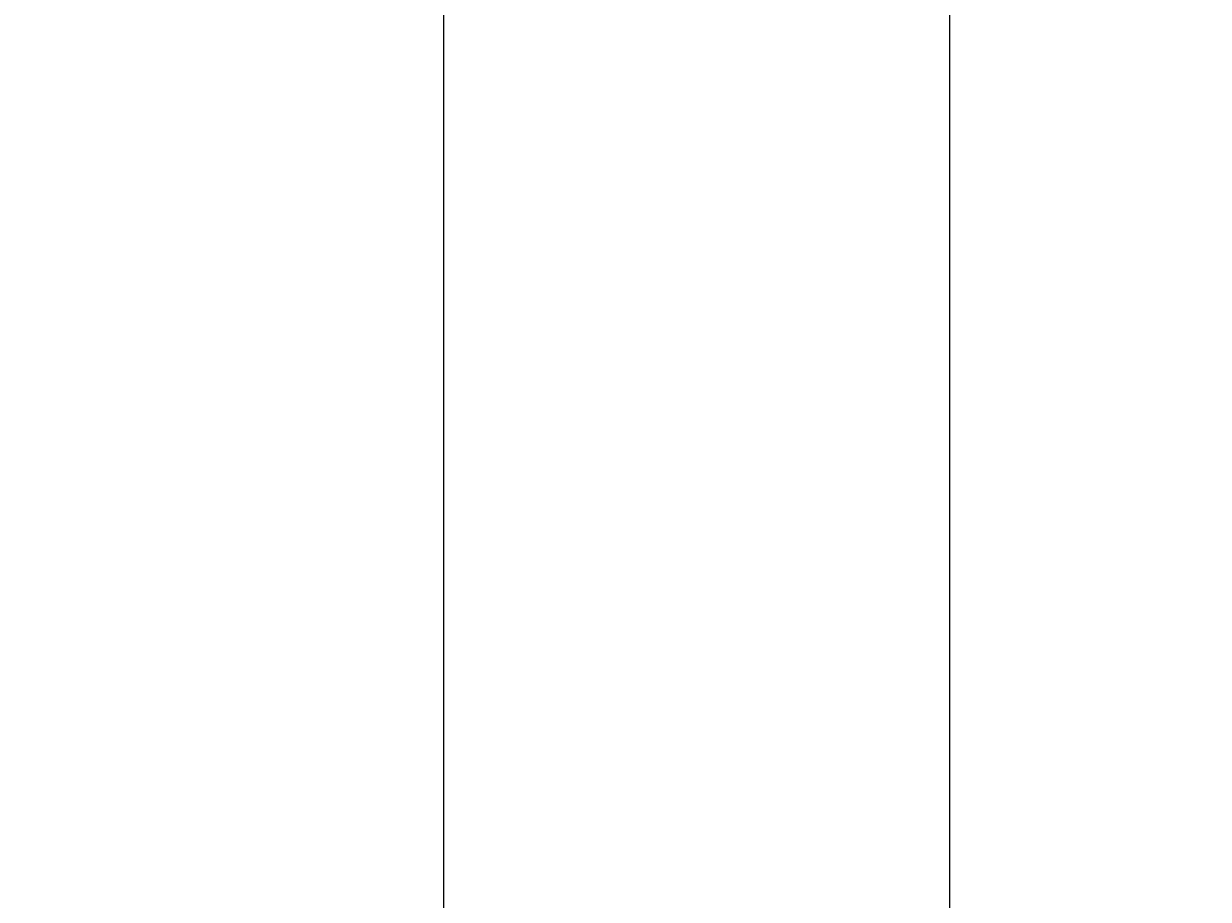
# Model space of a CAD drawing. Units: millimetres. Extents: x 19292 to 100733, y 12374 to 26974.
# Tile 6 of 24: x 29402 to 29589, y 15391 to 15530. Entities that reach past the tile are written whole.
import ezdxf

# ---------------------------------------------------------------- set-up
doc = ezdxf.new("R2010")
doc.units = ezdxf.units.MM
doc.layers.add('A-ANNO-DIMS', color=2, linetype='Continuous', lineweight=18)
doc.layers.add('A-DOOR', color=4, linetype='Continuous', lineweight=25)
doc.styles.get("Standard").update_dxf_attribs({"font": 'arial.ttf'})
doc.dimstyles.get("Standard").update_dxf_attribs({"dimtxt": 0.18, "dimasz": 0.18, "dimexe": 0.18, "dimexo": 0.0625, "dimgap": 0.09, "dimtad": 0, "dimtih": 1, "dimtoh": 1, "dimdec": 4, "dimzin": 0, "dimdsep": 46, "dimtxsty": 'Standard', "dimcen": 0.09, "dimadec": 0, "dimazin": 0, "dimtfac": 1, "dimtdec": 4, "dimtofl": 0, "dimtmove": 0, "dimatfit": 3, "dimfxl": 1, "dimtolj": 1, "dimtzin": 0, "dimarcsym": 0})

# ---------------------------------------------------------------- blocks, each defined once
blk = doc.blocks.new('*D79')
at = {"layer": 'A-ANNO-DIMS', "color": 0, "lineweight": -2, "transparency": 16777216}
for p, q in [((22694.13, 22860.66), (22694.13, 12808.81)), ((36144.17, 15985.66), (36144.17, 12808.81)), ((22694.31, 12808.99), (29418.73, 12808.99)), ((36143.99, 12808.99), (29419.57, 12808.99))]:
    blk.add_line(p, q, dxfattribs=at)
at = {"layer": 'A-ANNO-DIMS', "color": 0, "transparency": 16777216}
for points in [[(22694.31, 12809.02), (22694.31, 12808.96), (22694.13, 12808.99)], [(36143.99, 12809.02), (36143.99, 12808.96), (36144.17, 12808.99)]]:
    blk.add_solid(points, dxfattribs=at)
at = {"layer": 'Defpoints', "color": 0, "transparency": 16777216}
for p in [(22694.13, 22860.72), (36144.17, 15985.72), (36144.17, 12808.99)]:
    blk.add_point(p, dxfattribs=at)
at = {"layer": 'A-ANNO-DIMS', "color": 0, "transparency": 16777216, "insert": (29419.15, 12808.99), "char_height": 0.18, "attachment_point": 5}
blk.add_mtext('\\A1;13450', dxfattribs=at)
blk = doc.blocks.new('*D82')
at = {"layer": 'A-ANNO-DIMS', "color": 0, "lineweight": -2, "transparency": 16777216}
for p, q in [((27198.81, 13562.81), (27198.81, 23555.9)), ((27198.99, 23555.72), (29296.44, 23555.72)), ((31394.62, 23555.72), (29297.17, 23555.72)), ((31394.8, 13544.06), (31394.8, 23555.9))]:
    blk.add_line(p, q, dxfattribs=at)
at = {"layer": 'A-ANNO-DIMS', "color": 0, "transparency": 16777216}
for points in [[(27198.99, 23555.75), (27198.99, 23555.69), (27198.81, 23555.72)], [(31394.62, 23555.75), (31394.62, 23555.69), (31394.8, 23555.72)]]:
    blk.add_solid(points, dxfattribs=at)
at = {"layer": 'Defpoints', "color": 0, "transparency": 16777216}
for p in [(31394.8, 23555.72), (27198.81, 13562.75), (31394.8, 13543.99)]:
    blk.add_point(p, dxfattribs=at)
at = {"layer": 'A-ANNO-DIMS', "color": 0, "transparency": 16777216, "insert": (29296.81, 23555.72), "char_height": 0.18, "attachment_point": 5}
blk.add_mtext('\\A1;4196', dxfattribs=at)
blk = doc.blocks.new('*D86')
at = {"layer": 'A-ANNO-DIMS', "color": 0, "lineweight": -2, "transparency": 16777216}
for p, q in [((27198.81, 15132.81), (27198.81, 23555.9)), ((27198.99, 23555.72), (29198.45, 23555.72)), ((31198.63, 23555.72), (29199.18, 23555.72)), ((31198.81, 15132.81), (31198.81, 23555.9))]:
    blk.add_line(p, q, dxfattribs=at)
at = {"layer": 'A-ANNO-DIMS', "color": 0, "transparency": 16777216}
for points in [[(27198.99, 23555.75), (27198.99, 23555.69), (27198.81, 23555.72)], [(31198.63, 23555.75), (31198.63, 23555.69), (31198.81, 23555.72)]]:
    blk.add_solid(points, dxfattribs=at)
at = {"layer": 'Defpoints', "color": 0, "transparency": 16777216}
for p in [(31198.81, 23555.72), (27198.81, 15132.75), (31198.81, 15132.75)]:
    blk.add_point(p, dxfattribs=at)
at = {"layer": 'A-ANNO-DIMS', "color": 0, "transparency": 16777216, "insert": (29198.81, 23555.72), "char_height": 0.18, "attachment_point": 5}
blk.add_mtext('\\A1;4000', dxfattribs=at)

msp = doc.modelspace()

# ---------------------------------------------------------------- linework, layer by layer
at = {"layer": 'A-DOOR'}
for p, q in [((29468.571, 14906.403), (29468.571, 15641.675)), ((29548.571, 14906.403), (29548.571, 15641.675))]:
    msp.add_line(p, q, dxfattribs=at)
msp.add_arc((29468.571, 14906.403), 735.272, 0, 90, dxfattribs=at)

# ---------------------------------------------------------------- dimensions: what is measured, and where the dimension line sits
at = {"layer": 'A-ANNO-DIMS'}
for base, p1, p2, picture, middle in [((31394.799, 23555.725), (27198.815, 13562.748), (31394.799, 13543.993), '*D82', (29296.807, 23555.725)), ((31198.815, 23555.725), (27198.815, 15132.748), (31198.815, 15132.748), '*D86', (29198.815, 23555.725)), ((36144.169, 12808.993), (22694.132, 22860.725), (36144.169, 15985.725), '*D79', (29419.151, 12808.993))]:
    dim = msp.add_linear_dim(base=base, p1=p1, p2=p2, dimstyle='Standard', override={"dimdec": 0, "dimlfac": 1, "dimrnd": 0, "dimzin": 0, "dimdsep": 46, "dimlunit": 2}, dxfattribs=at)
    dim.commit()
    dim.dimension.update_dxf_attribs({"geometry": picture, "text_midpoint": middle})

doc.saveas('drawing.dxf')
